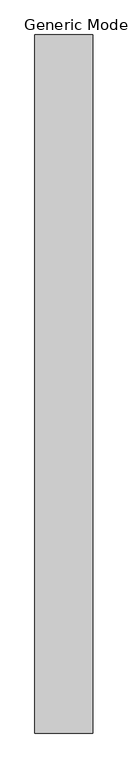
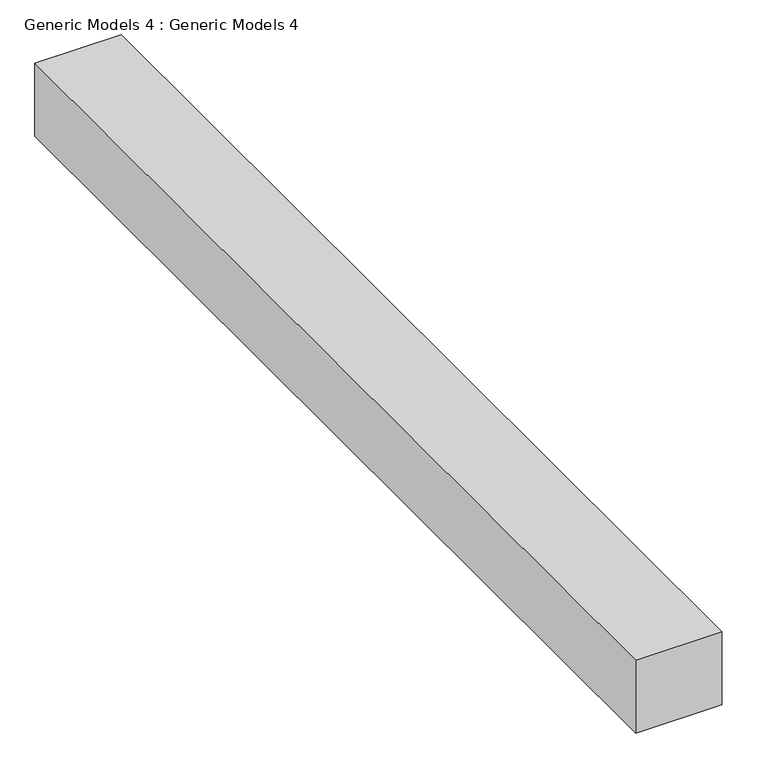
"""IFC4 building model written with IfcOpenShell, lengths in millimetres: proxy geometry, Generic Models 4 : Generic Models 4."""

from ifc_helpers import new_model, si_unit, frame, origin, place, context, project, spatial, polyline, outline, extrude, source, transform, mapped, element, save


def generic_models_4_generic_models_4_fc34fd45(model_context):
    return source(origin(), model_context, "Body", "SweptSolid", [
        extrude(outline(polyline([(-8586.8607234, -9739.3538163), (-8245.991855, -9739.3538163), (-8245.991855, -13854.1538163), (-8586.8607234, -13854.1538163), (-8586.8607234, -9739.3538163)])), frame((0.0, 0.0, 6400.8), z_axis=(0.0, 0.0, 1.0), x_axis=(1.0, 0.0, 0.0)), (0.0, 0.0, 1.0), 304.8),
    ])


if __name__ == "__main__":
    model = new_model("IFC4")
    model_context = context("Model", 3, world=origin())
    ifc_project = project(units=[si_unit("LENGTHUNIT", "METRE", prefix="MILLI")], contexts=[model_context])
    site = spatial("IfcSite", under=ifc_project)
    building = spatial("IfcBuilding", under=site)
    placement = place(None, origin())
    generic_models_4_generic_models_4_shape = generic_models_4_generic_models_4_fc34fd45(model_context)
    element("IfcBuildingElementProxy", 1, Name="Generic Models 4 : Generic Models 4", ObjectType="Generic Models 4 : Generic Models 4", at=placement, inside=building, context=model_context, shape_type="MappedRepresentation", body=[
        mapped(generic_models_4_generic_models_4_shape, transform((0.0, 0.0, 0.0), x_axis=(1.0, 0.0, 0.0), y_axis=(0.0, 1.0, 0.0), z_axis=(0.0, 0.0, 1.0))),
    ])
    save(model, "model.ifc")
